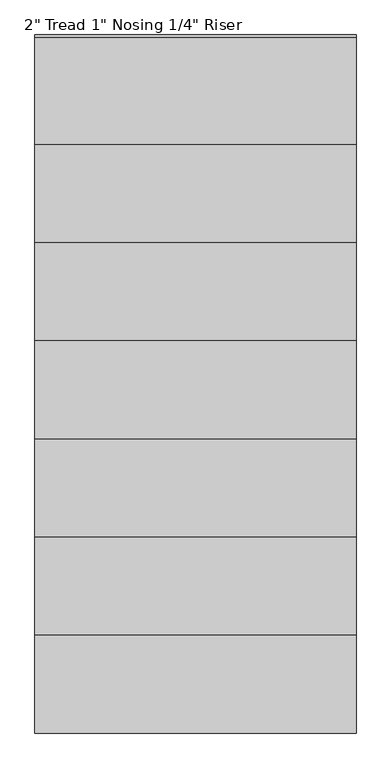
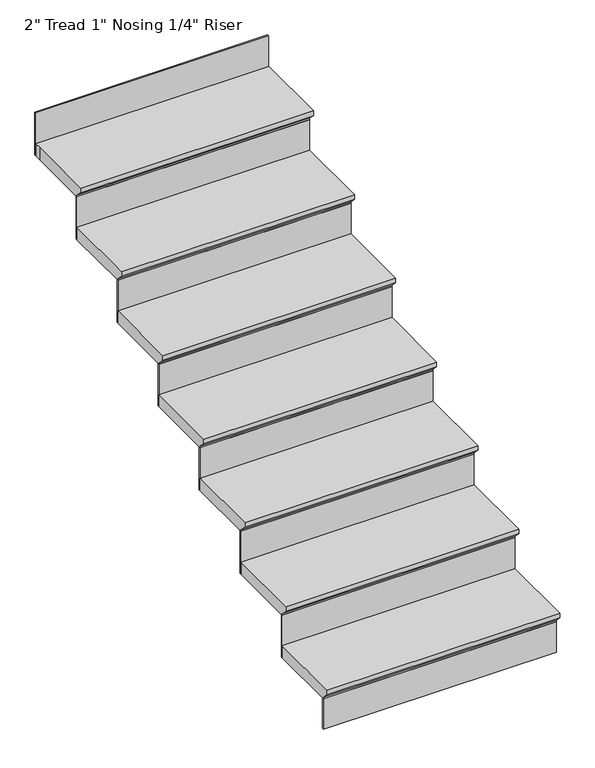
"""IFC4 building model written with IfcOpenShell, lengths in millimetres: stair flight geometry."""

from ifc_helpers import new_model, si_unit, origin, place, context, project, spatial, faceted_brep, source, transform, mapped, element, save


def stair_flight_d2e0b81c(model_context):
    return source(origin(), model_context, "Body", "Brep", [
        faceted_brep([(1046.3501403, 157.6257925, 768.35), (1046.3501403, 157.6257925, 787.4), (131.9501403, 157.6257925, 787.4), (131.9501403, 157.6257925, 768.35), (1046.3501403, 183.0257925, 742.95), (131.9501403, 183.0257925, 742.95), (1046.3501403, 462.4257925, 787.4), (131.9501403, 462.4257925, 787.4), (131.9501403, 183.0257925, 736.6), (131.9501403, 462.4257925, 736.6), (1046.3501403, 462.4257925, 736.6), (1046.3501403, 183.0257925, 736.6)], [[[0, 1, 2, 3]], [[4, 0, 3, 5]], [[2, 1, 6, 7]], [[8, 9, 10, 11]], [[2, 7, 9, 8, 5, 3]], [[8, 11, 4, 5]], [[6, 1, 0, 4, 11, 10]], [[7, 6, 10, 9]]]),
        faceted_brep([(1046.3501403, 183.0257925, 736.6), (1046.3501403, 183.0257925, 609.6), (1046.3501403, 189.3757925, 609.6), (1046.3501403, 189.3757925, 736.6), (131.9501403, 183.0257925, 736.6), (131.9501403, 189.3757925, 736.6), (131.9501403, 189.3757925, 609.6), (131.9501403, 183.0257925, 609.6)], [[[0, 1, 2, 3]], [[4, 5, 6, 7]], [[1, 0, 4, 7]], [[2, 1, 7, 6]], [[3, 2, 6, 5]], [[0, 3, 5, 4]]]),
        faceted_brep([(1046.3501403, 462.4257925, 914.4), (1046.3501403, 462.4257925, 736.6), (1046.3501403, 468.7757925, 736.6), (1046.3501403, 468.7757925, 914.4), (131.9501403, 462.4257925, 914.4), (131.9501403, 468.7757925, 914.4), (131.9501403, 468.7757925, 736.6), (131.9501403, 462.4257925, 736.6)], [[[0, 1, 2, 3]], [[4, 5, 6, 7]], [[1, 0, 4, 7]], [[2, 1, 7, 6]], [[3, 2, 6, 5]], [[0, 3, 5, 4]]]),
        faceted_brep([(131.9501403, 437.0257925, 965.2), (1046.3501403, 437.0257925, 965.2), (1046.3501403, 741.8257925, 965.2), (131.9501403, 741.8257925, 965.2), (131.9501403, 462.4257925, 914.4), (131.9501403, 741.8257925, 914.4), (1046.3501403, 741.8257925, 914.4), (1046.3501403, 462.4257925, 914.4), (131.9501403, 462.4257925, 920.75), (131.9501403, 437.0257925, 946.15), (1046.3501403, 462.4257925, 920.75), (1046.3501403, 437.0257925, 946.15)], [[[0, 1, 2, 3]], [[4, 5, 6, 7]], [[0, 3, 5, 4, 8, 9]], [[4, 7, 10, 8]], [[2, 1, 11, 10, 7, 6]], [[3, 2, 6, 5]], [[11, 1, 0, 9]], [[10, 11, 9, 8]]]),
        faceted_brep([(1046.3501403, 741.8257925, 1092.2), (1046.3501403, 741.8257925, 914.4), (1046.3501403, 748.1757925, 914.4), (1046.3501403, 748.1757925, 1092.2), (131.9501403, 741.8257925, 1092.2), (131.9501403, 748.1757925, 1092.2), (131.9501403, 748.1757925, 914.4), (131.9501403, 741.8257925, 914.4)], [[[0, 1, 2, 3]], [[4, 5, 6, 7]], [[1, 0, 4, 7]], [[2, 1, 7, 6]], [[3, 2, 6, 5]], [[0, 3, 5, 4]]]),
        faceted_brep([(131.9501403, 716.4257925, 1143.0), (1046.3501403, 716.4257925, 1143.0), (1046.3501403, 1021.2257925, 1143.0), (131.9501403, 1021.2257925, 1143.0), (131.9501403, 741.8257925, 1092.2), (131.9501403, 1021.2257925, 1092.2), (1046.3501403, 1021.2257925, 1092.2), (1046.3501403, 741.8257925, 1092.2), (131.9501403, 741.8257925, 1098.55), (131.9501403, 716.4257925, 1123.95), (1046.3501403, 741.8257925, 1098.55), (1046.3501403, 716.4257925, 1123.95)], [[[0, 1, 2, 3]], [[4, 5, 6, 7]], [[0, 3, 5, 4, 8, 9]], [[4, 7, 10, 8]], [[2, 1, 11, 10, 7, 6]], [[3, 2, 6, 5]], [[11, 1, 0, 9]], [[10, 11, 9, 8]]]),
        faceted_brep([(1046.3501403, 1021.2257925, 1270.0), (1046.3501403, 1021.2257925, 1092.2), (1046.3501403, 1027.5757925, 1092.2), (1046.3501403, 1027.5757925, 1270.0), (131.9501403, 1021.2257925, 1270.0), (131.9501403, 1027.5757925, 1270.0), (131.9501403, 1027.5757925, 1092.2), (131.9501403, 1021.2257925, 1092.2)], [[[0, 1, 2, 3]], [[4, 5, 6, 7]], [[1, 0, 4, 7]], [[2, 1, 7, 6]], [[3, 2, 6, 5]], [[0, 3, 5, 4]]]),
        faceted_brep([(131.9501403, 995.8257925, 1320.8), (1046.3501403, 995.8257925, 1320.8), (1046.3501403, 1300.6257925, 1320.8), (131.9501403, 1300.6257925, 1320.8), (131.9501403, 1021.2257925, 1270.0), (131.9501403, 1300.6257925, 1270.0), (1046.3501403, 1300.6257925, 1270.0), (1046.3501403, 1021.2257925, 1270.0), (131.9501403, 1021.2257925, 1276.35), (131.9501403, 995.8257925, 1301.75), (1046.3501403, 1021.2257925, 1276.35), (1046.3501403, 995.8257925, 1301.75)], [[[0, 1, 2, 3]], [[4, 5, 6, 7]], [[0, 3, 5, 4, 8, 9]], [[4, 7, 10, 8]], [[2, 1, 11, 10, 7, 6]], [[3, 2, 6, 5]], [[11, 1, 0, 9]], [[10, 11, 9, 8]]]),
        faceted_brep([(1046.3501403, 1300.6257925, 1447.8), (1046.3501403, 1300.6257925, 1270.0), (1046.3501403, 1306.9757925, 1270.0), (1046.3501403, 1306.9757925, 1447.8), (131.9501403, 1300.6257925, 1447.8), (131.9501403, 1306.9757925, 1447.8), (131.9501403, 1306.9757925, 1270.0), (131.9501403, 1300.6257925, 1270.0)], [[[0, 1, 2, 3]], [[4, 5, 6, 7]], [[1, 0, 4, 7]], [[2, 1, 7, 6]], [[3, 2, 6, 5]], [[0, 3, 5, 4]]]),
        faceted_brep([(131.9501403, 1275.2257925, 1498.6), (1046.3501403, 1275.2257925, 1498.6), (1046.3501403, 1580.0257925, 1498.6), (131.9501403, 1580.0257925, 1498.6), (131.9501403, 1300.6257925, 1447.8), (131.9501403, 1580.0257925, 1447.8), (1046.3501403, 1580.0257925, 1447.8), (1046.3501403, 1300.6257925, 1447.8), (131.9501403, 1300.6257925, 1454.15), (131.9501403, 1275.2257925, 1479.55), (1046.3501403, 1300.6257925, 1454.15), (1046.3501403, 1275.2257925, 1479.55)], [[[0, 1, 2, 3]], [[4, 5, 6, 7]], [[0, 3, 5, 4, 8, 9]], [[4, 7, 10, 8]], [[2, 1, 11, 10, 7, 6]], [[3, 2, 6, 5]], [[11, 1, 0, 9]], [[10, 11, 9, 8]]]),
        faceted_brep([(1046.3501403, 1580.0257925, 1625.6), (1046.3501403, 1580.0257925, 1447.8), (1046.3501403, 1586.3757925, 1447.8), (1046.3501403, 1586.3757925, 1625.6), (131.9501403, 1580.0257925, 1625.6), (131.9501403, 1586.3757925, 1625.6), (131.9501403, 1586.3757925, 1447.8), (131.9501403, 1580.0257925, 1447.8)], [[[0, 1, 2, 3]], [[4, 5, 6, 7]], [[1, 0, 4, 7]], [[2, 1, 7, 6]], [[3, 2, 6, 5]], [[0, 3, 5, 4]]]),
        faceted_brep([(131.9501403, 1554.6257925, 1676.4), (1046.3501403, 1554.6257925, 1676.4), (1046.3501403, 1859.4257925, 1676.4), (131.9501403, 1859.4257925, 1676.4), (131.9501403, 1580.0257925, 1625.6), (131.9501403, 1859.4257925, 1625.6), (1046.3501403, 1859.4257925, 1625.6), (1046.3501403, 1580.0257925, 1625.6), (131.9501403, 1580.0257925, 1631.95), (131.9501403, 1554.6257925, 1657.35), (1046.3501403, 1580.0257925, 1631.95), (1046.3501403, 1554.6257925, 1657.35)], [[[0, 1, 2, 3]], [[4, 5, 6, 7]], [[0, 3, 5, 4, 8, 9]], [[4, 7, 10, 8]], [[2, 1, 11, 10, 7, 6]], [[3, 2, 6, 5]], [[11, 1, 0, 9]], [[10, 11, 9, 8]]]),
        faceted_brep([(1046.3501403, 2138.8257925, 1981.2), (1046.3501403, 2138.8257925, 1803.4), (1046.3501403, 2145.1757925, 1803.4), (1046.3501403, 2145.1757925, 1981.2), (131.9501403, 2138.8257925, 1981.2), (131.9501403, 2145.1757925, 1981.2), (131.9501403, 2145.1757925, 1803.4), (131.9501403, 2138.8257925, 1803.4)], [[[0, 1, 2, 3]], [[4, 5, 6, 7]], [[1, 0, 4, 7]], [[2, 1, 7, 6]], [[3, 2, 6, 5]], [[0, 3, 5, 4]]]),
        faceted_brep([(1046.3501403, 1859.4257925, 1803.4), (1046.3501403, 1859.4257925, 1625.6), (1046.3501403, 1865.7757925, 1625.6), (1046.3501403, 1865.7757925, 1803.4), (131.9501403, 1859.4257925, 1803.4), (131.9501403, 1865.7757925, 1803.4), (131.9501403, 1865.7757925, 1625.6), (131.9501403, 1859.4257925, 1625.6)], [[[0, 1, 2, 3]], [[4, 5, 6, 7]], [[1, 0, 4, 7]], [[2, 1, 7, 6]], [[3, 2, 6, 5]], [[0, 3, 5, 4]]]),
        faceted_brep([(131.9501403, 2138.8257925, 1854.2), (131.9501403, 2113.4257925, 1854.2), (131.9501403, 1834.0257925, 1854.2), (1046.3501403, 1834.0257925, 1854.2), (1046.3501403, 2138.8257925, 1854.2), (131.9501403, 2113.4257925, 1803.4), (131.9501403, 2138.8257925, 1803.4), (1046.3501403, 2138.8257925, 1803.4), (1046.3501403, 1859.4257925, 1803.4), (131.9501403, 1859.4257925, 1803.4), (131.9501403, 1859.4257925, 1809.75), (131.9501403, 1834.0257925, 1835.15), (1046.3501403, 1859.4257925, 1809.75), (1046.3501403, 1834.0257925, 1835.15)], [[[0, 1, 2, 3, 4]], [[5, 6, 7, 8, 9]], [[1, 0, 6, 5]], [[2, 1, 5, 9, 10, 11]], [[9, 8, 12, 10]], [[4, 3, 13, 12, 8, 7]], [[0, 4, 7, 6]], [[13, 3, 2, 11]], [[12, 13, 11, 10]]]),
    ])


if __name__ == "__main__":
    model = new_model("IFC4")
    model_context = context("Model", 3, world=origin())
    ifc_project = project(units=[si_unit("LENGTHUNIT", "METRE", prefix="MILLI")], contexts=[model_context])
    site = spatial("IfcSite", under=ifc_project)
    building = spatial("IfcBuilding", under=site)
    placement = place(None, origin())
    stair_flight_shape = stair_flight_d2e0b81c(model_context)
    element("IfcStairFlight", 1, ObjectType="2\" Tread 1\" Nosing 1/4\" Riser", at=placement, inside=building, context=model_context, shape_type="MappedRepresentation", body=[
        mapped(stair_flight_shape, transform((0.0, 0.0, 0.0), x_axis=(1.0, 0.0, 0.0), y_axis=(0.0, 1.0, 0.0), z_axis=(0.0, 0.0, 1.0))),
    ])
    save(model, "model.ifc")
